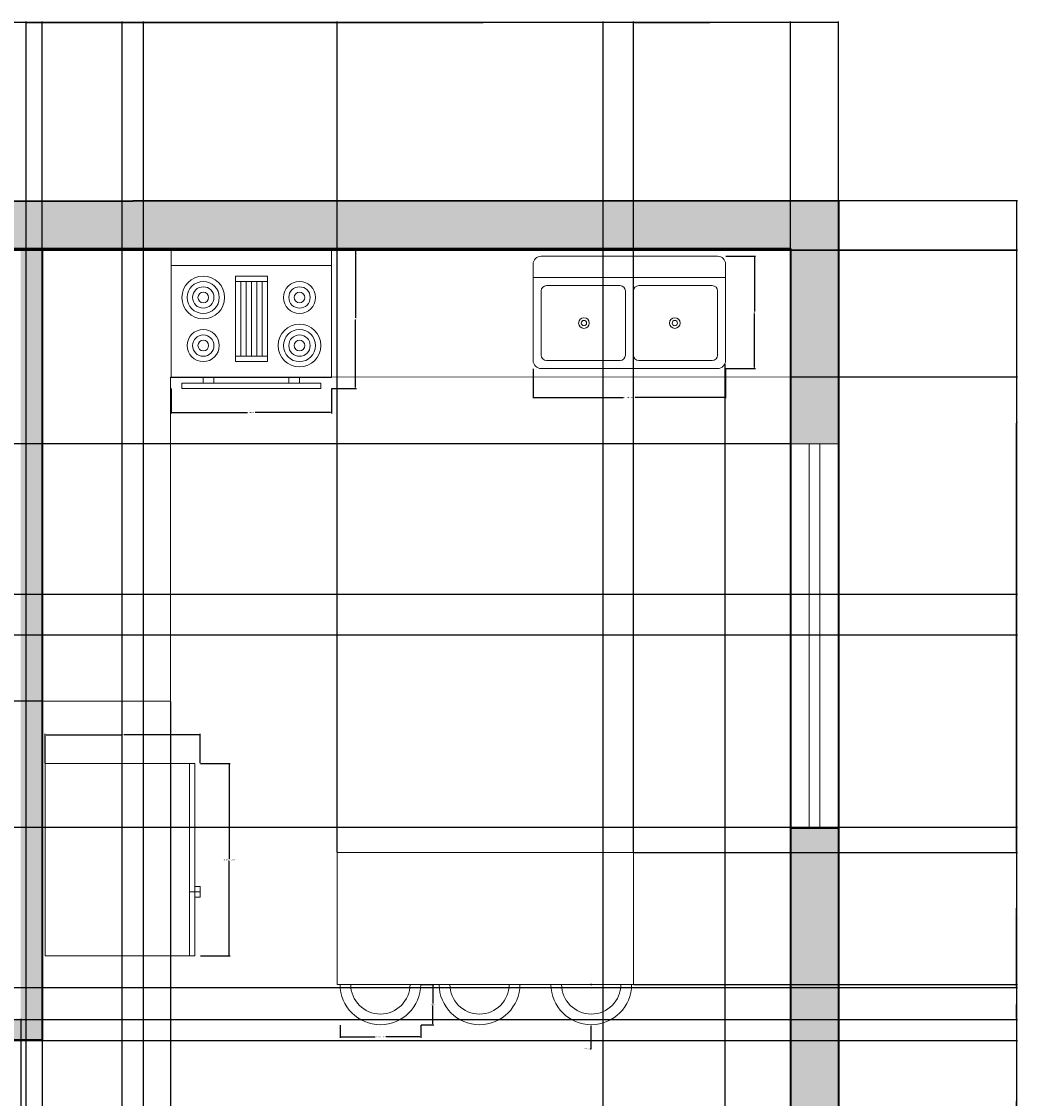
# Model space of a CAD drawing. Units: inches. Extents: x 1531 to 2263, y 2711 to 3216.
# Tile 12 of 12: x 2076 to 2263, y 3015 to 3216. Entities that reach past the tile are written whole.
import ezdxf

# ---------------------------------------------------------------- set-up
doc = ezdxf.new("R2010")
doc.units = ezdxf.units.IN
for name, color, linetype, lineweight in [('A-ANNO-DIMS', 2, 'Continuous', 18), ('A-EQPM', 8, 'Continuous', 18), ('A-FLOR-CASE', 9, 'Continuous', 18), ('A-FLOR-FIXT', 9, 'Continuous', 18), ('A-FURN', 8, 'Continuous', 18), ('A-GLAZ', 4, 'Continuous', 18), ('A-WALL', 7, 'Continuous', 35)]:
    doc.layers.add(name, color=color, linetype=linetype, lineweight=lineweight)
doc.layers.add('A-WALL-PATT', color=18, linetype='Continuous', lineweight=13, true_color=0x000000)
doc.styles.get("Standard").update_dxf_attribs({"font": 'arial.ttf'})
doc.dimstyles.get("Standard").update_dxf_attribs({"dimtxt": 0.18, "dimasz": 0.18, "dimexe": 0.18, "dimexo": 0.0625, "dimgap": 0.09, "dimtad": 0, "dimtih": 1, "dimtoh": 1, "dimdec": 4, "dimzin": 0, "dimdsep": 46, "dimtxsty": 'Standard', "dimcen": 0.09, "dimadec": 0, "dimazin": 0, "dimtfac": 1, "dimtdec": 4, "dimtofl": 0, "dimtmove": 0, "dimatfit": 3, "dimfxl": 1, "dimtolj": 1, "dimtzin": 0, "dimarcsym": 0})

# ---------------------------------------------------------------- blocks, each defined once
blk = doc.blocks.new('Range-Oven - 30 in top')
for p, q in [((0, -3), (30, -3)), ((12, -6), (18, -6)), ((13, -20), (13, -6)), ((14, -6), (14, -20)), ((15, -20), (15, -6)), ((16, -6), (16, -20)), ((17, -20), (17, -6)), ((18, -20), (12, -20)), ((6, -24), (6, -25)), ((8, -25), (8, -24)), ((22, -25), (22, -24)), ((24, -24), (24, -25))]:
    blk.add_line(p, q)
for points in [[(0, -24), (0, 0), (30, 0), (30, -24)], [(12, -21), (12, -5), (18, -5), (18, -21)], [(2, -26), (2, -25), (28, -25), (28, -26)]]:
    blk.add_lwpolyline(points, close=True)
for centre, radius in [((6, -9), 4), ((6, -9), 3), ((24, -9), 3), ((6, -9), 2), ((6, -9), 1), ((24, -9), 2), ((24, -9), 1), ((24, -18), 4), ((6, -18), 3), ((6, -18), 2), ((24, -18), 3), ((24, -18), 2), ((6, -18), 1), ((24, -18), 1)]:
    blk.add_circle(centre, radius)
blk = doc.blocks.new('Sink-double - 36 in top')
for p, q in [((-18, -4), (18, -4)), ((-0.75, -18.5), (-0.75, -6.5)), ((0.75, -6.5), (0.75, -18.5))]:
    blk.add_line(p, q)
for points in [[(-16.5, 0), (16.5, 0)], [(-18, -19.5), (-18, -1.5)], [(18, -1.5), (18, -19.5)], [(-15.5, -5.5), (-1.75, -5.5)], [(1.75, -5.5), (15.5, -5.5)], [(-16.5, -18.5), (-16.5, -6.5)], [(16.5, -6.5), (16.5, -18.5)], [(-1.75, -19.5), (-15.5, -19.5)], [(15.5, -19.5), (1.75, -19.5)], [(16.5, -21), (-16.5, -21)]]:
    blk.add_lwpolyline(points)
for centre, radius in [((-8.5, -12.5), 1), ((-8.5, -12.5), 0.5), ((8.5, -12.5), 1), ((8.5, -12.5), 0.5)]:
    blk.add_circle(centre, radius)
for centre, radius, start, end in [((-16.5, -1.5), 1.5, 90, 180), ((16.5, -1.5), 1.5, 0, 90), ((-15.5, -6.5), 1, 90, 180), ((-1.75, -6.5), 1, 0, 90), ((1.75, -6.5), 1, 90, 180), ((15.5, -6.5), 1, 0, 90), ((-16.5, -19.5), 1.5, 180, 270), ((-15.5, -18.5), 1, 180, 270), ((-1.75, -18.5), 1, 270, 0), ((1.75, -18.5), 1, 180, 270), ((15.5, -18.5), 1, 270, 0), ((16.5, -19.5), 1.5, 270, 0)]:
    blk.add_arc(centre, radius, start, end)
blk = doc.blocks.new('Refrigerator-2 door - 36 in top')
for p, q in [((0, -26.999999), (36, -26.999999)), ((11, -27.999999), (11, -28.999999)), ((12, -26.999999), (12, -28.999999)), ((13, -28.999999), (13, -27.999999)), ((11, -28.999999), (13, -28.999999))]:
    blk.add_line(p, q)
blk.add_lwpolyline([(0, -27.999999), (0, 0), (36, 0), (36, -27.999999)], close=True)
blk = doc.blocks.new('WIN-72IN')
for p, q in [((0, 5.5), (72, 5.5)), ((0, 3.5), (72, 3.5))]:
    blk.add_line(p, q)
for points in [[(0, 9), (0, 0)], [(72, 0), (72, 9)]]:
    blk.add_lwpolyline(points)
blk = doc.blocks.new('ISLAND-STOOL')
for radius in [7.55, 5.55]:
    blk.add_arc((7.55, 7.55), radius, 180, 0)
blk = doc.blocks.new('*D42')
at = {"layer": 'A-ANNO-DIMS', "color": 0, "lineweight": -2, "transparency": 16777216}
for p, q in [((2135.65, 3028.72), (2135.65, 3026.34)), ((2150.76, 3028.72), (2150.76, 3026.34)), ((2135.83, 3026.52), (2142.21, 3026.52)), ((2150.58, 3026.52), (2144.19, 3026.52))]:
    blk.add_line(p, q, dxfattribs=at)
at = {"layer": 'A-ANNO-DIMS', "color": 0, "transparency": 16777216}
for points in [[(2135.83, 3026.55), (2135.83, 3026.49), (2135.65, 3026.52)], [(2150.58, 3026.55), (2150.58, 3026.49), (2150.76, 3026.52)]]:
    blk.add_solid(points, dxfattribs=at)
at = {"layer": 'Defpoints', "color": 0, "transparency": 16777216}
for p in [(2135.65, 3028.78), (2150.76, 3028.78), (2150.76, 3026.52)]:
    blk.add_point(p, dxfattribs=at)
at = {"layer": 'A-ANNO-DIMS', "color": 0, "transparency": 16777216, "insert": (2143.2, 3026.52), "char_height": 0.18, "attachment_point": 5}
blk.add_mtext('\\A1;STOOL 15 TYP.', dxfattribs=at)
blk = doc.blocks.new('*D43')
at = {"layer": 'A-ANNO-DIMS', "color": 0, "lineweight": -2, "transparency": 16777216}
for p, q in [((2150.82, 3036.34), (2153.2, 3036.34)), ((2153.02, 3036.16), (2153.02, 3032.74)), ((2153.02, 3028.96), (2153.02, 3032.38)), ((2150.82, 3028.78), (2153.2, 3028.78))]:
    blk.add_line(p, q, dxfattribs=at)
at = {"layer": 'A-ANNO-DIMS', "color": 0, "transparency": 16777216}
for points in [[(2152.99, 3036.16), (2153.05, 3036.16), (2153.02, 3036.34)], [(2152.99, 3028.96), (2153.05, 3028.96), (2153.02, 3028.78)]]:
    blk.add_solid(points, dxfattribs=at)
at = {"layer": 'Defpoints', "color": 0, "transparency": 16777216}
for p in [(2150.76, 3036.34), (2153.02, 3036.34), (2150.76, 3028.78)]:
    blk.add_point(p, dxfattribs=at)
at = {"layer": 'A-ANNO-DIMS', "color": 0, "transparency": 16777216, "insert": (2153.02, 3032.56), "char_height": 0.18, "attachment_point": 5}
blk.add_mtext('\\A1;8 TYP.', dxfattribs=at)
blk = doc.blocks.new('*D46')
at = {"layer": 'A-ANNO-DIMS', "color": 0, "lineweight": -2, "transparency": 16777216}
for p, q in [((2104.07, 3147.79), (2104.07, 3143.17)), ((2134.07, 3147.79), (2134.07, 3143.17)), ((2104.25, 3143.35), (2118.37, 3143.35)), ((2133.89, 3143.35), (2119.77, 3143.35))]:
    blk.add_line(p, q, dxfattribs=at)
at = {"layer": 'A-ANNO-DIMS', "color": 0, "transparency": 16777216}
for points in [[(2104.25, 3143.38), (2104.25, 3143.32), (2104.07, 3143.35)], [(2133.89, 3143.38), (2133.89, 3143.32), (2134.07, 3143.35)]]:
    blk.add_solid(points, dxfattribs=at)
at = {"layer": 'Defpoints', "color": 0, "transparency": 16777216}
for p in [(2104.07, 3147.85), (2134.07, 3147.85), (2134.07, 3143.35)]:
    blk.add_point(p, dxfattribs=at)
at = {"layer": 'A-ANNO-DIMS', "color": 0, "transparency": 16777216, "insert": (2119.07, 3143.35), "char_height": 0.18, "attachment_point": 5}
blk.add_mtext('\\A1;RANGE 30', dxfattribs=at)
blk = doc.blocks.new('*D47')
at = {"layer": 'A-ANNO-DIMS', "color": 0, "lineweight": -2, "transparency": 16777216}
for p, q in [((2134.13, 3173.85), (2138.75, 3173.85)), ((2138.57, 3173.67), (2138.57, 3161.03)), ((2138.57, 3148.03), (2138.57, 3160.67)), ((2134.13, 3147.85), (2138.75, 3147.85))]:
    blk.add_line(p, q, dxfattribs=at)
at = {"layer": 'A-ANNO-DIMS', "color": 0, "transparency": 16777216}
for points in [[(2138.54, 3173.67), (2138.6, 3173.67), (2138.57, 3173.85)], [(2138.54, 3148.03), (2138.6, 3148.03), (2138.57, 3147.85)]]:
    blk.add_solid(points, dxfattribs=at)
at = {"layer": 'Defpoints', "color": 0, "transparency": 16777216}
for p in [(2134.07, 3173.85), (2138.57, 3173.85), (2134.07, 3147.85)]:
    blk.add_point(p, dxfattribs=at)
at = {"layer": 'A-ANNO-DIMS', "color": 0, "transparency": 16777216, "insert": (2138.57, 3160.85), "char_height": 0.18, "attachment_point": 5}
blk.add_mtext('\\A1;26', dxfattribs=at)
blk = doc.blocks.new('*D48')
at = {"layer": 'A-ANNO-DIMS', "color": 0, "lineweight": -2, "transparency": 16777216}
for p, q in [((2171.78, 3151.5), (2171.78, 3145.98)), ((2207.78, 3151.5), (2207.78, 3145.98)), ((2171.96, 3146.16), (2188.69, 3146.16)), ((2207.6, 3146.16), (2190.87, 3146.16))]:
    blk.add_line(p, q, dxfattribs=at)
at = {"layer": 'A-ANNO-DIMS', "color": 0, "transparency": 16777216}
for points in [[(2171.96, 3146.19), (2171.96, 3146.13), (2171.78, 3146.16)], [(2207.6, 3146.19), (2207.6, 3146.13), (2207.78, 3146.16)]]:
    blk.add_solid(points, dxfattribs=at)
at = {"layer": 'Defpoints', "color": 0, "transparency": 16777216}
for p in [(2171.78, 3151.56), (2207.78, 3151.56), (2207.78, 3146.16)]:
    blk.add_point(p, dxfattribs=at)
at = {"layer": 'A-ANNO-DIMS', "color": 0, "transparency": 16777216, "insert": (2189.78, 3146.16), "char_height": 0.18, "attachment_point": 5}
blk.add_mtext('\\A1;DOUBLE SINK 36', dxfattribs=at)
blk = doc.blocks.new('*D49')
at = {"layer": 'A-ANNO-DIMS', "color": 0, "lineweight": -2, "transparency": 16777216}
for p, q in [((2207.84, 3172.56), (2213.36, 3172.56)), ((2213.18, 3172.38), (2213.18, 3162.24)), ((2213.18, 3151.74), (2213.18, 3161.88)), ((2207.84, 3151.56), (2213.36, 3151.56))]:
    blk.add_line(p, q, dxfattribs=at)
at = {"layer": 'A-ANNO-DIMS', "color": 0, "transparency": 16777216}
for points in [[(2213.15, 3172.38), (2213.21, 3172.38), (2213.18, 3172.56)], [(2213.15, 3151.74), (2213.21, 3151.74), (2213.18, 3151.56)]]:
    blk.add_solid(points, dxfattribs=at)
at = {"layer": 'Defpoints', "color": 0, "transparency": 16777216}
for p in [(2207.78, 3172.56), (2213.18, 3172.56), (2207.78, 3151.56)]:
    blk.add_point(p, dxfattribs=at)
at = {"layer": 'A-ANNO-DIMS', "color": 0, "transparency": 16777216, "insert": (2213.18, 3162.06), "char_height": 0.18, "attachment_point": 5}
blk.add_mtext('\\A1;21', dxfattribs=at)
blk = doc.blocks.new('*D50')
at = {"layer": 'A-ANNO-DIMS', "color": 0, "lineweight": -2, "transparency": 16777216}
for p, q in [((2109.56, 3077.65), (2115.08, 3077.65)), ((2114.9, 3077.47), (2114.9, 3059.84)), ((2114.9, 3041.83), (2114.9, 3059.47)), ((2109.56, 3041.65), (2115.08, 3041.65))]:
    blk.add_line(p, q, dxfattribs=at)
at = {"layer": 'A-ANNO-DIMS', "color": 0, "transparency": 16777216}
for points in [[(2114.87, 3077.47), (2114.93, 3077.47), (2114.9, 3077.65)], [(2114.87, 3041.83), (2114.93, 3041.83), (2114.9, 3041.65)]]:
    blk.add_solid(points, dxfattribs=at)
at = {"layer": 'Defpoints', "color": 0, "transparency": 16777216}
for p in [(2109.5, 3077.65), (2114.9, 3077.65), (2109.5, 3041.65)]:
    blk.add_point(p, dxfattribs=at)
at = {"layer": 'A-ANNO-DIMS', "color": 0, "transparency": 16777216, "insert": (2114.9, 3059.65), "char_height": 0.18, "attachment_point": 5}
blk.add_mtext('\\A1;REFRIGERATOR 36', dxfattribs=at)
blk = doc.blocks.new('*D51')
at = {"layer": 'A-ANNO-DIMS', "color": 0, "lineweight": -2, "transparency": 16777216}
for p, q in [((2080.5, 3077.72), (2080.5, 3083.23)), ((2080.68, 3083.05), (2094.78, 3083.05)), ((2109.32, 3083.05), (2095.22, 3083.05)), ((2109.5, 3077.72), (2109.5, 3083.23))]:
    blk.add_line(p, q, dxfattribs=at)
at = {"layer": 'A-ANNO-DIMS', "color": 0, "transparency": 16777216}
for points in [[(2080.68, 3083.08), (2080.68, 3083.02), (2080.5, 3083.05)], [(2109.32, 3083.08), (2109.32, 3083.02), (2109.5, 3083.05)]]:
    blk.add_solid(points, dxfattribs=at)
at = {"layer": 'Defpoints', "color": 0, "transparency": 16777216}
for p in [(2080.5, 3083.05), (2080.5, 3077.65), (2109.5, 3077.65)]:
    blk.add_point(p, dxfattribs=at)
at = {"layer": 'A-ANNO-DIMS', "color": 0, "transparency": 16777216, "insert": (2095, 3083.05), "char_height": 0.18, "attachment_point": 5}
blk.add_mtext('\\A1;29', dxfattribs=at)
blk = doc.blocks.new('*D54')
at = {"layer": 'A-ANNO-DIMS', "color": 0, "lineweight": -2, "transparency": 16777216}
for p, q in [((1568.91, 3182.74), (1568.91, 3216.47)), ((1569.09, 3216.29), (1898.62, 3216.29)), ((2228.73, 3216.29), (1899.2, 3216.29)), ((2228.91, 3183.08), (2228.91, 3216.47))]:
    blk.add_line(p, q, dxfattribs=at)
at = {"layer": 'A-ANNO-DIMS', "color": 0, "transparency": 16777216}
for points in [[(1569.09, 3216.32), (1569.09, 3216.26), (1568.91, 3216.29)], [(2228.73, 3216.32), (2228.73, 3216.26), (2228.91, 3216.29)]]:
    blk.add_solid(points, dxfattribs=at)
at = {"layer": 'Defpoints', "color": 0, "transparency": 16777216}
for p in [(2228.91, 3216.29), (1568.91, 3182.67), (2228.91, 3183.02)]:
    blk.add_point(p, dxfattribs=at)
at = {"layer": 'A-ANNO-DIMS', "color": 0, "transparency": 16777216, "insert": (1898.91, 3216.29), "char_height": 0.18, "attachment_point": 5}
blk.add_mtext('\\A1;660', dxfattribs=at)
blk = doc.blocks.new('*D55')
at = {"layer": 'A-ANNO-DIMS', "color": 0, "lineweight": -2, "transparency": 16777216}
for p, q in [((2228.97, 3183.02), (2262.37, 3183.02)), ((2262.19, 3182.84), (2262.19, 2963.95)), ((2262.19, 2744.7), (2262.19, 2963.59)), ((2076.3, 2744.52), (2262.37, 2744.52))]:
    blk.add_line(p, q, dxfattribs=at)
at = {"layer": 'A-ANNO-DIMS', "color": 0, "transparency": 16777216}
for points in [[(2262.16, 3182.84), (2262.22, 3182.84), (2262.19, 3183.02)], [(2262.16, 2744.7), (2262.22, 2744.7), (2262.19, 2744.52)]]:
    blk.add_solid(points, dxfattribs=at)
at = {"layer": 'Defpoints', "color": 0, "transparency": 16777216}
for p in [(2228.91, 3183.02), (2076.24, 2744.52), (2262.19, 2744.52)]:
    blk.add_point(p, dxfattribs=at)
at = {"layer": 'A-ANNO-DIMS', "color": 0, "transparency": 16777216, "insert": (2262.19, 2963.77), "char_height": 0.18, "attachment_point": 5}
blk.add_mtext('\\A1;438.5', dxfattribs=at)
blk = doc.blocks.new('*D62')
at = {"layer": 'A-ANNO-DIMS', "color": 0, "lineweight": -2, "transparency": 16777216}
for p, q in [((2079.91, 3174), (2079.91, 3216.47)), ((2080.09, 3216.29), (2149.63, 3216.29)), ((2219.73, 3216.29), (2150.19, 3216.29)), ((2219.91, 3174.08), (2219.91, 3216.47))]:
    blk.add_line(p, q, dxfattribs=at)
at = {"layer": 'A-ANNO-DIMS', "color": 0, "transparency": 16777216}
for points in [[(2080.09, 3216.32), (2080.09, 3216.26), (2079.91, 3216.29)], [(2219.73, 3216.32), (2219.73, 3216.26), (2219.91, 3216.29)]]:
    blk.add_solid(points, dxfattribs=at)
at = {"layer": 'Defpoints', "color": 0, "transparency": 16777216}
for p in [(2219.91, 3216.29), (2079.91, 3173.94), (2219.91, 3174.02)]:
    blk.add_point(p, dxfattribs=at)
at = {"layer": 'A-ANNO-DIMS', "color": 0, "transparency": 16777216, "insert": (2149.91, 3216.29), "char_height": 0.18, "attachment_point": 5}
blk.add_mtext('\\A1;140', dxfattribs=at)
blk = doc.blocks.new('*D76')
at = {"layer": 'A-ANNO-DIMS', "color": 0, "lineweight": -2, "transparency": 16777216}
for p, q in [((2094.87, 2975.39), (2094.87, 3216.47)), ((2095.05, 3216.29), (2139.65, 3216.29)), ((2184.69, 3216.29), (2140.09, 3216.29)), ((2184.87, 2975.44), (2184.87, 3216.47))]:
    blk.add_line(p, q, dxfattribs=at)
at = {"layer": 'A-ANNO-DIMS', "color": 0, "transparency": 16777216}
for points in [[(2095.05, 3216.32), (2095.05, 3216.26), (2094.87, 3216.29)], [(2184.69, 3216.32), (2184.69, 3216.26), (2184.87, 3216.29)]]:
    blk.add_solid(points, dxfattribs=at)
at = {"layer": 'Defpoints', "color": 0, "transparency": 16777216}
for p in [(2184.87, 3216.29), (2094.87, 2975.33), (2184.87, 2975.38)]:
    blk.add_point(p, dxfattribs=at)
at = {"layer": 'A-ANNO-DIMS', "color": 0, "transparency": 16777216, "insert": (2139.87, 3216.29), "char_height": 0.18, "attachment_point": 5}
blk.add_mtext('\\A1;90', dxfattribs=at)
blk = doc.blocks.new('*D80')
at = {"layer": 'A-ANNO-DIMS', "color": 0, "lineweight": -2, "transparency": 16777216}
for p, q in [((1715.97, 3173.75), (2262.37, 3173.75)), ((2262.19, 3173.57), (2262.19, 3137.93)), ((2262.19, 3101.93), (2262.19, 3137.57)), ((1715.97, 3101.75), (2262.37, 3101.75))]:
    blk.add_line(p, q, dxfattribs=at)
at = {"layer": 'A-ANNO-DIMS', "color": 0, "transparency": 16777216}
for points in [[(2262.16, 3173.57), (2262.22, 3173.57), (2262.19, 3173.75)], [(2262.16, 3101.93), (2262.22, 3101.93), (2262.19, 3101.75)]]:
    blk.add_solid(points, dxfattribs=at)
at = {"layer": 'Defpoints', "color": 0, "transparency": 16777216}
for p in [(1715.91, 3173.75), (1715.91, 3101.75), (2262.19, 3101.75)]:
    blk.add_point(p, dxfattribs=at)
at = {"layer": 'A-ANNO-DIMS', "color": 0, "transparency": 16777216, "insert": (2262.19, 3137.75), "char_height": 0.18, "attachment_point": 5}
blk.add_mtext('\\A1;72', dxfattribs=at)
blk = doc.blocks.new('*D82')
at = {"layer": 'A-ANNO-DIMS', "color": 0, "lineweight": -2, "transparency": 16777216}
for p, q in [((2135.09, 3061.07), (2135.09, 3216.47)), ((2135.27, 3216.29), (2162.42, 3216.29)), ((2190.37, 3216.29), (2163.21, 3216.29)), ((2190.55, 3061.07), (2190.55, 3216.47))]:
    blk.add_line(p, q, dxfattribs=at)
at = {"layer": 'A-ANNO-DIMS', "color": 0, "transparency": 16777216}
for points in [[(2135.27, 3216.32), (2135.27, 3216.26), (2135.09, 3216.29)], [(2190.37, 3216.32), (2190.37, 3216.26), (2190.55, 3216.29)]]:
    blk.add_solid(points, dxfattribs=at)
at = {"layer": 'Defpoints', "color": 0, "transparency": 16777216}
for p in [(2190.55, 3216.29), (2135.09, 3061.01), (2190.55, 3061.01)]:
    blk.add_point(p, dxfattribs=at)
at = {"layer": 'A-ANNO-DIMS', "color": 0, "transparency": 16777216, "insert": (2162.82, 3216.29), "char_height": 0.18, "attachment_point": 5}
blk.add_mtext('\\A1;55.46', dxfattribs=at)
blk = doc.blocks.new('*D83')
at = {"layer": 'A-ANNO-DIMS', "color": 0, "lineweight": -2, "transparency": 16777216}
for p, q in [((2190.61, 3061.01), (2262.37, 3061.01)), ((2262.19, 3060.83), (2262.19, 3048.86)), ((2262.19, 3036.52), (2262.19, 3048.49)), ((2190.61, 3036.34), (2262.37, 3036.34))]:
    blk.add_line(p, q, dxfattribs=at)
at = {"layer": 'A-ANNO-DIMS', "color": 0, "transparency": 16777216}
for points in [[(2262.16, 3060.83), (2262.22, 3060.83), (2262.19, 3061.01)], [(2262.16, 3036.52), (2262.22, 3036.52), (2262.19, 3036.34)]]:
    blk.add_solid(points, dxfattribs=at)
at = {"layer": 'Defpoints', "color": 0, "transparency": 16777216}
for p in [(2190.55, 3061.01), (2190.55, 3036.34), (2262.19, 3036.34)]:
    blk.add_point(p, dxfattribs=at)
at = {"layer": 'A-ANNO-DIMS', "color": 0, "transparency": 16777216, "insert": (2262.19, 3048.67), "char_height": 0.18, "attachment_point": 5}
blk.add_mtext('\\A1;24.674', dxfattribs=at)
blk = doc.blocks.new('*D84')
at = {"layer": 'A-ANNO-DIMS', "color": 0, "lineweight": -2, "transparency": 16777216}
for p, q in [((2079.91, 3089.28), (2079.91, 2711.06)), ((2103.91, 3089.28), (2103.91, 2711.06)), ((2080.09, 2711.24), (2091.69, 2711.24)), ((2103.73, 2711.24), (2092.13, 2711.24))]:
    blk.add_line(p, q, dxfattribs=at)
at = {"layer": 'A-ANNO-DIMS', "color": 0, "transparency": 16777216}
for points in [[(2080.09, 2711.27), (2080.09, 2711.21), (2079.91, 2711.24)], [(2103.73, 2711.27), (2103.73, 2711.21), (2103.91, 2711.24)]]:
    blk.add_solid(points, dxfattribs=at)
at = {"layer": 'Defpoints', "color": 0, "transparency": 16777216}
for p in [(2079.91, 3089.34), (2103.91, 3089.34), (2103.91, 2711.24)]:
    blk.add_point(p, dxfattribs=at)
at = {"layer": 'A-ANNO-DIMS', "color": 0, "transparency": 16777216, "insert": (2091.91, 2711.24), "char_height": 0.18, "attachment_point": 5}
blk.add_mtext('\\A1;24', dxfattribs=at)
blk = doc.blocks.new('*D85')
at = {"layer": 'A-ANNO-DIMS', "color": 0, "lineweight": -2, "transparency": 16777216}
for p, q in [((2079.85, 3173.94), (1531.04, 3173.94)), ((1531.22, 3173.76), (1531.22, 3131.82)), ((1531.22, 3089.52), (1531.22, 3131.46)), ((2079.85, 3089.34), (1531.04, 3089.34))]:
    blk.add_line(p, q, dxfattribs=at)
at = {"layer": 'A-ANNO-DIMS', "color": 0, "transparency": 16777216}
for points in [[(1531.19, 3173.76), (1531.25, 3173.76), (1531.22, 3173.94)], [(1531.19, 3089.52), (1531.25, 3089.52), (1531.22, 3089.34)]]:
    blk.add_solid(points, dxfattribs=at)
at = {"layer": 'Defpoints', "color": 0, "transparency": 16777216}
for p in [(1531.22, 3173.94), (2079.91, 3173.94), (2079.91, 3089.34)]:
    blk.add_point(p, dxfattribs=at)
at = {"layer": 'A-ANNO-DIMS', "color": 0, "transparency": 16777216, "insert": (1531.22, 3131.64), "char_height": 0.18, "attachment_point": 5}
blk.add_mtext('\\A1;84.6', dxfattribs=at)
blk = doc.blocks.new('*D86')
at = {"layer": 'A-ANNO-DIMS', "color": 0, "lineweight": -2, "transparency": 16777216}
for p, q in [((1715.97, 3065.75), (2262.37, 3065.75)), ((2262.19, 3065.57), (2262.19, 3050.93)), ((2262.19, 3035.93), (2262.19, 3050.57)), ((1715.97, 3035.75), (2262.37, 3035.75))]:
    blk.add_line(p, q, dxfattribs=at)
at = {"layer": 'A-ANNO-DIMS', "color": 0, "transparency": 16777216}
for points in [[(2262.16, 3065.57), (2262.22, 3065.57), (2262.19, 3065.75)], [(2262.16, 3035.93), (2262.22, 3035.93), (2262.19, 3035.75)]]:
    blk.add_solid(points, dxfattribs=at)
at = {"layer": 'Defpoints', "color": 0, "transparency": 16777216}
for p in [(1715.91, 3065.75), (2262.19, 3065.75), (1715.91, 3035.75)]:
    blk.add_point(p, dxfattribs=at)
at = {"layer": 'A-ANNO-DIMS', "color": 0, "transparency": 16777216, "insert": (2262.19, 3050.75), "char_height": 0.18, "attachment_point": 5}
blk.add_mtext('\\A1;30', dxfattribs=at)
blk = doc.blocks.new('*D100')
at = {"layer": 'A-ANNO-DIMS', "color": 0, "lineweight": -2, "transparency": 16777216}
for p, q in [((2219.85, 3174.02), (1531.04, 3174.02)), ((1531.22, 3173.84), (1531.22, 3155.93)), ((1531.22, 3137.67), (1531.22, 3155.57)), ((2219.85, 3137.49), (1531.04, 3137.49))]:
    blk.add_line(p, q, dxfattribs=at)
at = {"layer": 'A-ANNO-DIMS', "color": 0, "transparency": 16777216}
for points in [[(1531.19, 3173.84), (1531.25, 3173.84), (1531.22, 3174.02)], [(1531.19, 3137.67), (1531.25, 3137.67), (1531.22, 3137.49)]]:
    blk.add_solid(points, dxfattribs=at)
at = {"layer": 'Defpoints', "color": 0, "transparency": 16777216}
for p in [(2219.91, 3174.02), (1531.22, 3137.49), (2219.91, 3137.49)]:
    blk.add_point(p, dxfattribs=at)
at = {"layer": 'A-ANNO-DIMS', "color": 0, "transparency": 16777216, "insert": (1531.22, 3155.75), "char_height": 0.18, "attachment_point": 5}
blk.add_mtext('\\A1;36.526', dxfattribs=at)
blk = doc.blocks.new('*D103')
at = {"layer": 'A-ANNO-DIMS', "color": 0, "lineweight": -2, "transparency": 16777216}
for p, q in [((1577.97, 3173.68), (2262.37, 3173.68)), ((2262.19, 3173.5), (2262.19, 3141.71)), ((2262.19, 3109.55), (2262.19, 3141.34)), ((1577.97, 3109.37), (2262.37, 3109.37))]:
    blk.add_line(p, q, dxfattribs=at)
at = {"layer": 'A-ANNO-DIMS', "color": 0, "transparency": 16777216}
for points in [[(2262.16, 3173.5), (2262.22, 3173.5), (2262.19, 3173.68)], [(2262.16, 3109.55), (2262.22, 3109.55), (2262.19, 3109.37)]]:
    blk.add_solid(points, dxfattribs=at)
at = {"layer": 'Defpoints', "color": 0, "transparency": 16777216}
for p in [(1577.91, 3173.68), (1577.91, 3109.37), (2262.19, 3109.37)]:
    blk.add_point(p, dxfattribs=at)
at = {"layer": 'A-ANNO-DIMS', "color": 0, "transparency": 16777216, "insert": (2262.19, 3141.52), "char_height": 0.18, "attachment_point": 5}
blk.add_mtext('\\A1;64.31', dxfattribs=at)
blk = doc.blocks.new('*D106')
at = {"layer": 'A-ANNO-DIMS', "color": 0, "lineweight": -2, "transparency": 16777216}
for p, q in [((2190.55, 3061.07), (2190.55, 3216.47)), ((2190.73, 3216.29), (2204.83, 3216.29)), ((2219.73, 3216.29), (2205.62, 3216.29)), ((2219.91, 3065.55), (2219.91, 3216.47))]:
    blk.add_line(p, q, dxfattribs=at)
at = {"layer": 'A-ANNO-DIMS', "color": 0, "transparency": 16777216}
for points in [[(2190.73, 3216.32), (2190.73, 3216.26), (2190.55, 3216.29)], [(2219.73, 3216.32), (2219.73, 3216.26), (2219.91, 3216.29)]]:
    blk.add_solid(points, dxfattribs=at)
at = {"layer": 'Defpoints', "color": 0, "transparency": 16777216}
for p in [(2219.91, 3216.29), (2219.91, 3065.49), (2190.55, 3061.01)]:
    blk.add_point(p, dxfattribs=at)
at = {"layer": 'A-ANNO-DIMS', "color": 0, "transparency": 16777216, "insert": (2205.23, 3216.29), "char_height": 0.18, "attachment_point": 5}
blk.add_mtext('\\A1;29.36', dxfattribs=at)
blk = doc.blocks.new('*D107')
at = {"layer": 'A-ANNO-DIMS', "color": 0, "lineweight": -2, "transparency": 16777216}
for p, q in [((2219.99, 3150.02), (2262.37, 3150.02)), ((2262.19, 3149.84), (2262.19, 3105.69)), ((2262.19, 3061.19), (2262.19, 3105.33)), ((2190.61, 3061.01), (2262.37, 3061.01))]:
    blk.add_line(p, q, dxfattribs=at)
at = {"layer": 'A-ANNO-DIMS', "color": 0, "transparency": 16777216}
for points in [[(2262.16, 3149.84), (2262.22, 3149.84), (2262.19, 3150.02)], [(2262.16, 3061.19), (2262.22, 3061.19), (2262.19, 3061.01)]]:
    blk.add_solid(points, dxfattribs=at)
at = {"layer": 'Defpoints', "color": 0, "transparency": 16777216}
for p in [(2219.92, 3150.02), (2262.19, 3150.02), (2190.55, 3061.01)]:
    blk.add_point(p, dxfattribs=at)
at = {"layer": 'A-ANNO-DIMS', "color": 0, "transparency": 16777216, "insert": (2262.19, 3105.51), "char_height": 0.18, "attachment_point": 5}
blk.add_mtext('\\A1;89', dxfattribs=at)
blk = doc.blocks.new('*D110')
at = {"layer": 'A-ANNO-DIMS', "color": 0, "lineweight": -2, "transparency": 16777216}
for p, q in [((1711.97, 3035.75), (2262.37, 3035.75)), ((2262.19, 3035.57), (2262.19, 3032.93)), ((2262.19, 3029.93), (2262.19, 3032.57)), ((1711.97, 3029.75), (2262.37, 3029.75))]:
    blk.add_line(p, q, dxfattribs=at)
at = {"layer": 'A-ANNO-DIMS', "color": 0, "transparency": 16777216}
for points in [[(2262.16, 3035.57), (2262.22, 3035.57), (2262.19, 3035.75)], [(2262.16, 3029.93), (2262.22, 3029.93), (2262.19, 3029.75)]]:
    blk.add_solid(points, dxfattribs=at)
at = {"layer": 'Defpoints', "color": 0, "transparency": 16777216}
for p in [(1711.91, 3035.75), (2262.19, 3035.75), (1711.91, 3029.75)]:
    blk.add_point(p, dxfattribs=at)
at = {"layer": 'A-ANNO-DIMS', "color": 0, "transparency": 16777216, "insert": (2262.19, 3032.75), "char_height": 0.18, "attachment_point": 5}
blk.add_mtext('\\A1;6', dxfattribs=at)
blk = doc.blocks.new('*D116')
at = {"layer": 'A-ANNO-DIMS', "color": 0, "lineweight": -2, "transparency": 16777216}
for p, q in [((1899.97, 3025.85), (2262.37, 3025.85)), ((2262.19, 3025.67), (2262.19, 3014.79)), ((2262.19, 3003.56), (2262.19, 3014.43)), ((1894.62, 3003.38), (2262.37, 3003.38))]:
    blk.add_line(p, q, dxfattribs=at)
at = {"layer": 'A-ANNO-DIMS', "color": 0, "transparency": 16777216}
for points in [[(2262.16, 3025.67), (2262.22, 3025.67), (2262.19, 3025.85)], [(2262.16, 3003.56), (2262.22, 3003.56), (2262.19, 3003.38)]]:
    blk.add_solid(points, dxfattribs=at)
at = {"layer": 'Defpoints', "color": 0, "transparency": 16777216}
for p in [(1899.91, 3025.85), (1894.55, 3003.38), (2262.19, 3003.38)]:
    blk.add_point(p, dxfattribs=at)
at = {"layer": 'A-ANNO-DIMS', "color": 0, "transparency": 16777216, "insert": (2262.19, 3014.61), "char_height": 0.18, "attachment_point": 5}
blk.add_mtext('\\A1;22.47', dxfattribs=at)
blk = doc.blocks.new('*D121')
at = {"layer": 'A-ANNO-DIMS', "color": 0, "lineweight": -2, "transparency": 16777216}
for p, q in [((2052, 2979.08), (2052, 3216.47)), ((2052.18, 3216.29), (2073.04, 3216.29)), ((2094.69, 3216.29), (2073.83, 3216.29)), ((2094.87, 2979.39), (2094.87, 3216.47))]:
    blk.add_line(p, q, dxfattribs=at)
at = {"layer": 'A-ANNO-DIMS', "color": 0, "transparency": 16777216}
for points in [[(2052.18, 3216.32), (2052.18, 3216.26), (2052, 3216.29)], [(2094.69, 3216.32), (2094.69, 3216.26), (2094.87, 3216.29)]]:
    blk.add_solid(points, dxfattribs=at)
at = {"layer": 'Defpoints', "color": 0, "transparency": 16777216}
for p in [(2094.87, 3216.29), (2052, 2979.01), (2094.87, 2979.33)]:
    blk.add_point(p, dxfattribs=at)
at = {"layer": 'A-ANNO-DIMS', "color": 0, "transparency": 16777216, "insert": (2073.43, 3216.29), "char_height": 0.18, "attachment_point": 5}
blk.add_mtext('\\A1;42.87', dxfattribs=at)
blk = doc.blocks.new('*D123')
at = {"layer": 'A-ANNO-DIMS', "color": 0, "lineweight": -2, "transparency": 16777216}
for p, q in [((2207.66, 3152.42), (2207.66, 2711.06)), ((2219.92, 3149.95), (2219.92, 2711.06)), ((2207.84, 2711.24), (2213.41, 2711.24)), ((2219.74, 2711.24), (2214.18, 2711.24))]:
    blk.add_line(p, q, dxfattribs=at)
at = {"layer": 'A-ANNO-DIMS', "color": 0, "transparency": 16777216}
for points in [[(2207.84, 2711.27), (2207.84, 2711.21), (2207.66, 2711.24)], [(2219.74, 2711.27), (2219.74, 2711.21), (2219.92, 2711.24)]]:
    blk.add_solid(points, dxfattribs=at)
at = {"layer": 'Defpoints', "color": 0, "transparency": 16777216}
for p in [(2207.66, 3152.48), (2219.92, 3150.02), (2207.66, 2711.24)]:
    blk.add_point(p, dxfattribs=at)
at = {"layer": 'A-ANNO-DIMS', "color": 0, "transparency": 16777216, "insert": (2213.79, 2711.24), "char_height": 0.18, "attachment_point": 5}
blk.add_mtext('\\A1;12.26', dxfattribs=at)
blk = doc.blocks.new('*D124')
at = {"layer": 'A-ANNO-DIMS', "color": 0, "lineweight": -2, "transparency": 16777216}
for p, q in [((2076.91, 2862.01), (2076.91, 3216.47)), ((2077.09, 3216.29), (2087.69, 3216.29)), ((2098.73, 3216.29), (2088.13, 3216.29)), ((2098.91, 2862.01), (2098.91, 3216.47))]:
    blk.add_line(p, q, dxfattribs=at)
at = {"layer": 'A-ANNO-DIMS', "color": 0, "transparency": 16777216}
for points in [[(2077.09, 3216.32), (2077.09, 3216.26), (2076.91, 3216.29)], [(2098.73, 3216.32), (2098.73, 3216.26), (2098.91, 3216.29)]]:
    blk.add_solid(points, dxfattribs=at)
at = {"layer": 'Defpoints', "color": 0, "transparency": 16777216}
for p in [(2076.91, 3216.29), (2076.91, 2861.95), (2098.91, 2861.95)]:
    blk.add_point(p, dxfattribs=at)
at = {"layer": 'A-ANNO-DIMS', "color": 0, "transparency": 16777216, "insert": (2087.91, 3216.29), "char_height": 0.18, "attachment_point": 5}
blk.add_mtext('\\A1;22', dxfattribs=at)
blk = doc.blocks.new('*D130')
at = {"layer": 'A-ANNO-DIMS', "color": 0, "lineweight": -2, "transparency": 16777216}
for p, q in [((2075.91, 3029.88), (2075.91, 2711.06)), ((2079.91, 3025.88), (2079.91, 2711.06)), ((2076.09, 2711.24), (2077.76, 2711.24)), ((2079.73, 2711.24), (2078.06, 2711.24))]:
    blk.add_line(p, q, dxfattribs=at)
at = {"layer": 'A-ANNO-DIMS', "color": 0, "transparency": 16777216}
for points in [[(2076.09, 2711.27), (2076.09, 2711.21), (2075.91, 2711.24)], [(2079.73, 2711.27), (2079.73, 2711.21), (2079.91, 2711.24)]]:
    blk.add_solid(points, dxfattribs=at)
at = {"layer": 'Defpoints', "color": 0, "transparency": 16777216}
for p in [(2075.91, 3029.94), (2079.91, 3025.94), (2075.91, 2711.24)]:
    blk.add_point(p, dxfattribs=at)
at = {"layer": 'A-ANNO-DIMS', "color": 0, "transparency": 16777216, "insert": (2077.91, 2711.24), "char_height": 0.18, "attachment_point": 5}
blk.add_mtext('\\A1;4', dxfattribs=at)
blk = doc.blocks.new('*D134')
at = {"layer": 'A-ANNO-DIMS', "color": 0, "lineweight": -2, "transparency": 16777216}
for p, q in [((2182.65, 3036.25), (2182.65, 3036.43)), ((2182.56, 3036.34), (2182.74, 3036.34)), ((2182.65, 3024.25), (2182.65, 3028.6)), ((2182.47, 3024.25), (2182.65, 3024.25))]:
    blk.add_line(p, q, dxfattribs=at)
at = {"layer": 'A-ANNO-DIMS', "color": 0, "transparency": 16777216}
blk.add_solid([(2182.62, 3028.6), (2182.68, 3028.6), (2182.65, 3028.78)], dxfattribs=at)
at = {"layer": 'Defpoints', "color": 0, "transparency": 16777216}
for p in [(2182.65, 3036.34), (2182.65, 3028.78)]:
    blk.add_point(p, dxfattribs=at)
at = {"layer": 'A-ANNO-DIMS', "color": 0, "transparency": 16777216, "insert": (2181.8, 3024.25), "char_height": 0.18, "attachment_point": 5}
blk.add_mtext('\\A1;3X R7.553', dxfattribs=at)

msp = doc.modelspace()

# ---------------------------------------------------------------- hatches: boundary and pattern name
at = {"layer": 'A-WALL-PATT'}
h = msp.add_hatch(color=256, dxfattribs=at)
h.dxf.hatch_style = 1
h.paths.add_polyline_path([(2228.9101, 3183.02), (2055.9596, 3182.9296), (2055.9596, 3173.9296), (2075.9101, 3173.94), (2075.9101, 3029.94), (1959.9101, 3029.8793), (1959.9101, 3035.8772), (1955.9101, 3035.8772), (1955.9101, 3025.8772), (2079.9101, 3025.9421), (2079.9101, 3173.9421), (2219.9101, 3174.0153), (2219.9101, 3137.4897), (2228.9101, 3137.4897)])
h = msp.add_hatch(color=256, dxfattribs=at)
h.dxf.hatch_style = 1
h.paths.add_polyline_path([(2228.9101, 3065.4897), (2219.9101, 3065.4897), (2219.9101, 3026.0153), (2219.9101, 2979.3969), (2213.9101, 2979.3937), (2213.9101, 2975.3937), (2219.9101, 2975.3969), (2219.9101, 2966.8056), (2228.9101, 2966.8056)])

# ---------------------------------------------------------------- linework, layer by layer
at = {"layer": 'A-FLOR-CASE'}
for p, q in [((2109.0403, 3173.8485), (2109.0403, 3173.9573)), ((2103.9101, 3149.9546), (2219.9227, 3150.0153)), ((2103.9101, 3149.9546), (2103.9101, 3089.343)), ((2103.9101, 3089.343), (2079.9101, 3089.343))]:
    msp.add_line(p, q, dxfattribs=at)
msp.add_lwpolyline([(2135.086, 3061.0105), (2190.5472, 3061.0105), (2190.5472, 3036.3364), (2135.086, 3036.3364)], close=True, dxfattribs=at)
at = {"layer": 'A-WALL'}
for p, q in [((2079.9101, 3173.9421), (2219.9101, 3174.0153)), ((2079.9101, 3173.9421), (2079.9101, 3025.9421)), ((2219.9101, 3174.0153), (2219.9101, 3026.0153)), ((2219.9101, 3030.0153), (2219.9854, 3030.0153)), ((1955.9101, 3025.8772), (2079.9101, 3025.9421)), ((2219.9101, 3026.0153), (2219.9101, 2979.3969)), ((2219.9101, 3026.0153), (2219.9875, 3026.0153))]:
    msp.add_line(p, q, dxfattribs=at)
msp.add_lwpolyline([(1933.9101, 2762.8657), (1568.9111, 2762.6748), (1568.9111, 3182.6749), (2228.9101, 3183.02), (2228.9101, 2798.8631)], dxfattribs=at)

# ---------------------------------------------------------------- block references
at = {"layer": 'A-EQPM'}
msp.add_blockref('Range-Oven - 30 in top', (2104.0703, 3173.8485), dxfattribs=at)
at = {"layer": 'A-EQPM', "rotation": 90}
msp.add_blockref('Refrigerator-2 door - 36 in top', (2080.5021, 3041.6534), dxfattribs=at)
at = {"layer": 'A-FLOR-FIXT'}
msp.add_blockref('Sink-double - 36 in top', (2189.78, 3172.5616), dxfattribs=at)
at = {"layer": 'A-FURN'}
for p in [(2135.65, 3028.784), (2154.1948, 3028.784), (2175.0962, 3028.784)]:
    msp.add_blockref('ISLAND-STOOL', p, dxfattribs=at)
at = {"layer": 'A-GLAZ', "rotation": 269.9999999999999}
msp.add_blockref('WIN-72IN', (2219.9101, 3137.4896), dxfattribs=at)

# ---------------------------------------------------------------- dimensions: what is measured, and where the dimension line sits
at = {"layer": 'A-ANNO-DIMS'}
for base, p1, p2, override, picture, middle in [((2228.9101, 3216.295), (1568.9111, 3182.6749), (2228.9101, 3183.02), {"dimdec": 0, "dimlfac": 1, "dimrnd": 0, "dimzin": 0, "dimdsep": 46, "dimlunit": 2}, '*D54', (1898.9106, 3216.295)), ((2094.8704, 3216.295), (2051.9983, 2979.0128), (2094.8704, 2979.3315), {"dimdec": 2, "dimlfac": 1, "dimrnd": 0, "dimzin": 0, "dimdsep": 46, "dimlunit": 2}, '*D121', (2073.4343, 3216.295)), ((2076.9101, 3216.295), (2098.9101, 2861.9499), (2076.9101, 2861.9499), {"dimdec": 0, "dimlfac": 1, "dimrnd": 0, "dimzin": 0, "dimdsep": 46, "dimlunit": 2}, '*D124', (2087.9101, 3216.295)), ((2219.9101, 3216.295), (2079.9101, 3173.9421), (2219.9101, 3174.0153), {"dimdec": 0, "dimlfac": 1, "dimrnd": 0, "dimzin": 0, "dimdsep": 46, "dimlunit": 2}, '*D62', (2149.9101, 3216.295)), ((2184.8725, 3216.295), (2094.8725, 2975.3315), (2184.8725, 2975.3785), {"dimdec": 0, "dimlfac": 1, "dimrnd": 0, "dimzin": 0, "dimdsep": 46, "dimlunit": 2}, '*D76', (2139.8725, 3216.295)), ((2190.5472, 3216.295), (2135.086, 3061.0105), (2190.5472, 3061.0105), {"dimdec": 2, "dimlfac": 1, "dimrnd": 0, "dimzin": 0, "dimdsep": 46, "dimlunit": 2}, '*D82', (2162.8166, 3216.295)), ((2219.9101, 3216.295), (2190.5472, 3061.0105), (2219.9101, 3065.4897), {"dimdec": 2, "dimlfac": 1, "dimrnd": 0, "dimzin": 0, "dimdsep": 46, "dimlunit": 2}, '*D106', (2205.2287, 3216.295)), ((2207.6621, 2711.2407), (2219.9227, 3150.0153), (2207.6621, 3152.4778), {"dimdec": 2, "dimlfac": 1, "dimrnd": 0, "dimzin": 0, "dimdsep": 46, "dimlunit": 2}, '*D123', (2213.7924, 2711.2407)), ((2103.9101, 2711.2407), (2079.9101, 3089.343), (2103.9101, 3089.343), {"dimdec": 0, "dimlfac": 1, "dimrnd": 0, "dimzin": 0, "dimdsep": 46, "dimlunit": 2}, '*D84', (2091.9101, 2711.2407)), ((2075.9101, 2711.2407), (2079.9101, 3025.9421), (2075.9101, 3029.94), {"dimdec": 0, "dimlfac": 1, "dimrnd": 0, "dimzin": 0, "dimdsep": 46, "dimlunit": 2}, '*D130', (2077.9101, 2711.2407))]:
    dim = msp.add_linear_dim(base=base, p1=p1, p2=p2, dimstyle='Standard', override=override, dxfattribs=at)
    dim.commit()
    dim.dimension.update_dxf_attribs({"geometry": picture, "text_midpoint": middle})
for base, p1, p2, angle, override, picture, middle in [((2262.1851, 2744.5157), (2228.9101, 3183.02), (2076.2365, 2744.5157), 90, {"dimdec": 1, "dimlfac": 1, "dimrnd": 0, "dimzin": 0, "dimdsep": 46, "dimlunit": 2}, '*D55', (2262.1851, 2963.7678)), ((1531.2212, 3137.4897), (2219.9101, 3174.0153), (2219.9101, 3137.4897), 90, {"dimdec": 3, "dimlfac": 1, "dimrnd": 0, "dimzin": 0, "dimdsep": 46, "dimlunit": 2}, '*D100', (1531.2212, 3155.7525)), ((1531.2212, 3173.9421), (2079.9101, 3089.343), (2079.9101, 3173.9421), 90, {"dimdec": 1, "dimlfac": 1, "dimrnd": 0, "dimzin": 0, "dimdsep": 46, "dimlunit": 2}, '*D85', (1531.2212, 3131.6425)), ((2262.1851, 3109.3695), (1577.9111, 3173.6796), (1577.9111, 3109.3695), 90, {"dimdec": 2, "dimlfac": 1, "dimrnd": 0, "dimzin": 0, "dimdsep": 46, "dimlunit": 2}, '*D103', (2262.1851, 3141.5245)), ((2262.1851, 3101.7517), (1715.9101, 3173.7517), (1715.9101, 3101.7517), 90, {"dimdec": 0, "dimlfac": 1, "dimrnd": 0, "dimzin": 0, "dimdsep": 46, "dimlunit": 2}, '*D80', (2262.1851, 3137.7517)), ((2138.5703, 3173.8485), (2134.0703, 3147.8485), (2134.0703, 3173.8485), 90, {"dimdec": 0, "dimlfac": 1, "dimrnd": 0, "dimzin": 0, "dimdsep": 46, "dimlunit": 2}, '*D47', (2138.5703, 3160.8485)), ((2213.18, 3172.5616), (2207.78, 3151.5616), (2207.78, 3172.5616), 90, {"dimdec": 0, "dimlfac": 1, "dimrnd": 0, "dimzin": 0, "dimdsep": 46, "dimlunit": 2}, '*D49', (2213.18, 3162.0616)), ((2262.1851, 3150.0153), (2190.5472, 3061.0105), (2219.9227, 3150.0153), 90, {"dimdec": 0, "dimlfac": 1, "dimrnd": 0, "dimzin": 0, "dimdsep": 46, "dimlunit": 2}, '*D107', (2262.1851, 3105.5129)), ((2080.5021, 3083.0534), (2109.5021, 3077.6534), (2080.5021, 3077.6534), 180, {"dimdec": 0, "dimlfac": 1, "dimrnd": 0, "dimzin": 0, "dimdsep": 46, "dimlunit": 2}, '*D51', (2095.0021, 3083.0534)), ((2262.1851, 3065.7517), (1715.9101, 3035.7517), (1715.9101, 3065.7517), 90, {"dimdec": 0, "dimlfac": 1, "dimrnd": 0, "dimzin": 0, "dimdsep": 46, "dimlunit": 2}, '*D86', (2262.1851, 3050.7517)), ((2262.1851, 3036.3364), (2190.5472, 3061.0105), (2190.5472, 3036.3364), 90, {"dimdec": 3, "dimlfac": 1, "dimrnd": 0, "dimzin": 0, "dimdsep": 46, "dimlunit": 2}, '*D83', (2262.1851, 3048.6735)), ((2262.1851, 3035.7496), (1711.9101, 3029.7496), (1711.9101, 3035.7496), 90, {"dimdec": 0, "dimlfac": 1, "dimrnd": 0, "dimzin": 0, "dimdsep": 46, "dimlunit": 2}, '*D110', (2262.1851, 3032.7496)), ((2262.1851, 3003.376), (1899.9101, 3025.8479), (1894.5532, 3003.376), 90, {"dimdec": 2, "dimlfac": 1, "dimrnd": 0, "dimzin": 0, "dimdsep": 46, "dimlunit": 2}, '*D116', (2262.1851, 3014.6119))]:
    dim = msp.add_linear_dim(base=base, p1=p1, p2=p2, angle=angle, dimstyle='Standard', override=override, dxfattribs=at)
    dim.commit()
    dim.dimension.update_dxf_attribs({"geometry": picture, "text_midpoint": middle})
for base, p1, p2, text, picture, middle in [((2207.78, 3146.1616), (2171.78, 3151.5616), (2207.78, 3151.5616), 'DOUBLE SINK <>', '*D48', (2189.78, 3146.1616)), ((2134.0703, 3143.3485), (2104.0703, 3147.8485), (2134.0703, 3147.8485), 'RANGE <>', '*D46', (2119.0703, 3143.3485)), ((2150.7561, 3026.5177), (2135.6503, 3028.7836), (2150.7561, 3028.7836), 'STOOL <> TYP.', '*D42', (2143.2032, 3026.5177))]:
    dim = msp.add_linear_dim(base=base, p1=p1, p2=p2, text=text, dimstyle='Standard', override={"dimdec": 0, "dimlfac": 1, "dimrnd": 0, "dimzin": 0, "dimdsep": 46, "dimlunit": 2}, dxfattribs=at)
    dim.commit()
    dim.dimension.update_dxf_attribs({"geometry": picture, "text_midpoint": middle})
for base, p1, p2, text, picture, middle in [((2114.9021, 3077.6534), (2109.5021, 3041.6534), (2109.5021, 3077.6534), 'REFRIGERATOR <>', '*D50', (2114.9021, 3059.6534)), ((2153.0219, 3036.3364), (2150.7561, 3028.7836), (2150.7561, 3036.3364), '<> TYP.', '*D43', (2153.0219, 3032.56))]:
    dim = msp.add_linear_dim(base=base, p1=p1, p2=p2, angle=90, text=text, dimstyle='Standard', override={"dimdec": 0, "dimlfac": 1, "dimrnd": 0, "dimzin": 0, "dimdsep": 46, "dimlunit": 2}, dxfattribs=at)
    dim.commit()
    dim.dimension.update_dxf_attribs({"geometry": picture, "text_midpoint": middle})
dim = msp.add_radius_dim(center=(2182.6494, 3036.3364), mpoint=(2182.649, 3028.7836), text='3X <>', dimstyle='Standard', override={"dimdec": 3, "dimlfac": 1, "dimrnd": 0, "dimzin": 0, "dimdsep": 46, "dimlunit": 2}, dxfattribs=at)
dim.commit()
dim.dimension.update_dxf_attribs({"geometry": '*D134', "text_midpoint": (2181.7956, 3024.2519), "dimtype": 164})

doc.saveas('drawing.dxf')
